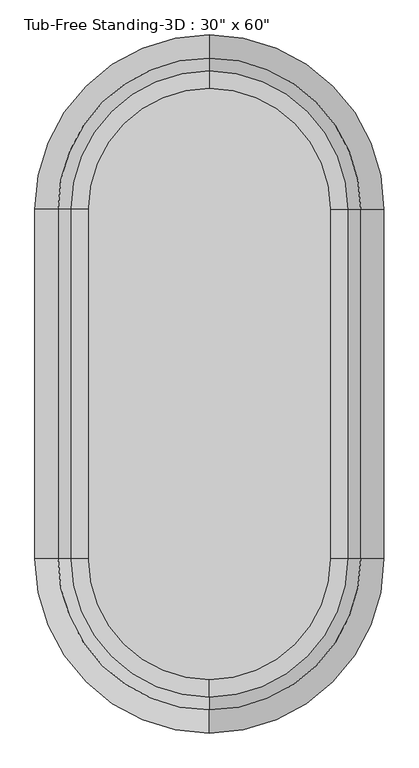
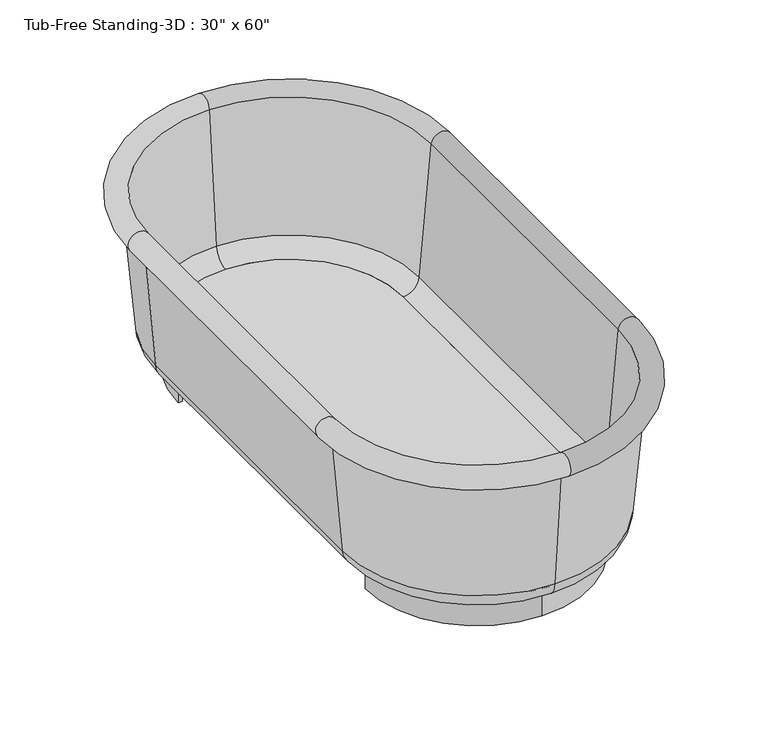
"""IFC4 building model written with IfcOpenShell, lengths in millimetres: flow terminal geometry."""

from ifc_helpers import new_model, si_unit, point, frame, frame_2d, origin, origin_with_axes, place, context, project, spatial, polyline, circle_curve, ellipse_curve, trimmed, segment, composite_curve, outline, extrude, source, transform, mapped, element, save
from ifc_brep_helpers import plane_surface, cylinder_surface, revolved_surface, advanced_brep


def flow_terminal_0c5ffde2(model_context):
    return source(origin(), model_context, "Body", "SolidModel", [
        advanced_brep(
        [(0.0, -723.9, 406.4), (342.9, -381.0, 406.4), (355.6, -381.0, 406.4), (0.0, -736.6, 406.4), (0.0, -698.1045038, 111.5561295), (317.1045038, -381.0, 111.5561295), (0.0, -645.2824236, 63.1536107), (264.2824236, -381.0, 63.1536107), (0.0, -645.2824236, 78.0774627), (264.2824236, -381.0, 78.0774627), (0.0, -683.2374416, 112.8568289), (302.2374416, -381.0, 112.8568289), (0.0, -711.4561556, 435.3982063), (330.4561556, -381.0, 435.3982063), (-342.9, -381.0, 406.4), (-355.6, -381.0, 406.4), (-317.1045038, -381.0, 111.5561295), (-264.2824236, -381.0, 63.1536107), (-264.2824236, -381.0, 78.0774627), (-302.2374416, -381.0, 112.8568289), (-330.4561556, -381.0, 435.3982063), (-355.6, 381.0, 406.4), (-342.9, 381.0, 406.4), (-317.1045038, 381.0, 111.5561295), (-264.2824236, 381.0, 63.1536107), (-264.2824236, 381.0, 78.0774627), (-302.2374416, 381.0, 112.8568289), (-330.4561556, 381.0, 435.3982063), (0.0, 723.9, 406.4), (0.0, 736.6, 406.4), (0.0, 698.1045038, 111.5561295), (0.0, 645.2824236, 63.1536107), (0.0, 645.2824236, 78.0774627), (0.0, 683.2374416, 112.8568289), (0.0, 711.4561556, 435.3982063), (342.9, 381.0, 406.4), (355.6, 381.0, 406.4), (317.1045038, 381.0, 111.5561295), (264.2824236, 381.0, 63.1536107), (264.2824236, 381.0, 78.0774627), (302.2374416, 381.0, 112.8568289), (330.4561556, 381.0, 435.3982063)],
        [
            (0, 1, circle_curve(frame((0.0, -381.0, 406.4), z_axis=(0.0, 0.0, 1.0), x_axis=(1.0, 0.0, 0.0)), 342.9)),
            (1, 2),
            (2, 3, circle_curve(frame((0.0, -381.0, 406.4), z_axis=(0.0, 0.0, -1.0), x_axis=(1.0, 0.0, 0.0)), 355.6)),
            (3, 0),
            (4, 5, circle_curve(frame((0.0, -381.0, 111.5561295), z_axis=(0.0, 0.0, 1.0), x_axis=(1.0, 0.0, 0.0)), 317.1045038)),
            (5, 1),
            (0, 4),
            (6, 7, circle_curve(frame((0.0, -381.0, 63.1536107), z_axis=(0.0, 0.0, 1.0), x_axis=(1.0, 0.0, 0.0)), 264.2824236)),
            (7, 5, circle_curve(frame((264.2824236, -381.0, 116.1774627), z_axis=(0.0, -1.0, 0.0), x_axis=(1.0, 0.0, 0.0)), 53.023852)),
            (4, 6, circle_curve(frame((0.0, -645.2824236, 116.1774627), z_axis=(1.0, 0.0, 0.0), x_axis=(0.0, -1.0, 0.0)), 53.023852)),
            (8, 9, circle_curve(frame((0.0, -381.0, 78.0774627), z_axis=(0.0, 0.0, 1.0), x_axis=(1.0, 0.0, 0.0)), 264.2824236)),
            (9, 7),
            (6, 8),
            (10, 11, circle_curve(frame((0.0, -381.0, 112.8568289), z_axis=(0.0, 0.0, 1.0), x_axis=(1.0, 0.0, 0.0)), 302.2374416)),
            (11, 9, circle_curve(frame((264.2824236, -381.0, 116.1774627), z_axis=(0.0, 1.0, 0.0), x_axis=(1.0, 0.0, 0.0)), 38.1)),
            (8, 10, circle_curve(frame((0.0, -645.2824236, 116.1774627), z_axis=(-1.0, 0.0, 0.0), x_axis=(0.0, -1.0, 0.0)), 38.1)),
            (12, 13, circle_curve(frame((0.0, -381.0, 435.3982063), z_axis=(0.0, 0.0, 1.0), x_axis=(1.0, 0.0, 0.0)), 330.4561556)),
            (13, 11),
            (10, 12),
            (2, 13, circle_curve(frame((355.6, -381.0, 431.8), z_axis=(0.0, -1.0, 0.0), x_axis=(1.0, 0.0, 0.0)), 25.4)),
            (12, 3, circle_curve(frame((0.0, -736.6, 431.8), z_axis=(1.0, 0.0, 0.0), x_axis=(0.0, -1.0, 0.0)), 25.4)),
            (14, 0, circle_curve(frame((0.0, -381.0, 406.4), z_axis=(0.0, 0.0, 1.0), x_axis=(0.0, -1.0, 0.0)), 342.9)),
            (3, 15, circle_curve(frame((0.0, -381.0, 406.4), z_axis=(0.0, 0.0, -1.0), x_axis=(0.0, -1.0, 0.0)), 355.6)),
            (15, 14),
            (16, 4, circle_curve(frame((0.0, -381.0, 111.5561295), z_axis=(0.0, 0.0, 1.0), x_axis=(0.0, -1.0, 0.0)), 317.1045038)),
            (14, 16),
            (17, 6, circle_curve(frame((0.0, -381.0, 63.1536107), z_axis=(0.0, 0.0, 1.0), x_axis=(0.0, -1.0, 0.0)), 264.2824236)),
            (16, 17, circle_curve(frame((-264.2824236, -381.0, 116.1774627), z_axis=(0.0, -1.0, 0.0), x_axis=(-1.0, 0.0, 0.0)), 53.023852)),
            (18, 8, circle_curve(frame((0.0, -381.0, 78.0774627), z_axis=(0.0, 0.0, 1.0), x_axis=(0.0, -1.0, 0.0)), 264.2824236)),
            (17, 18),
            (19, 10, circle_curve(frame((0.0, -381.0, 112.8568289), z_axis=(0.0, 0.0, 1.0), x_axis=(0.0, -1.0, 0.0)), 302.2374416)),
            (18, 19, circle_curve(frame((-264.2824236, -381.0, 116.1774627), z_axis=(0.0, 1.0, 0.0), x_axis=(-1.0, 0.0, 0.0)), 38.1)),
            (20, 12, circle_curve(frame((0.0, -381.0, 435.3982063), z_axis=(0.0, 0.0, 1.0), x_axis=(0.0, -1.0, 0.0)), 330.4561556)),
            (19, 20),
            (20, 15, circle_curve(frame((-355.6, -381.0, 431.8), z_axis=(0.0, -1.0, 0.0), x_axis=(-1.0, 0.0, 0.0)), 25.4)),
            (15, 21),
            (21, 22),
            (22, 14),
            (22, 23),
            (23, 16),
            (23, 24, circle_curve(frame((-264.2824236, 381.0, 116.1774627), z_axis=(0.0, -1.0, 0.0), x_axis=(-1.0, 0.0, 0.0)), 53.023852)),
            (24, 17),
            (24, 25),
            (25, 18),
            (25, 26, circle_curve(frame((-264.2824236, 381.0, 116.1774627), z_axis=(0.0, 1.0, 0.0), x_axis=(-1.0, 0.0, 0.0)), 38.1)),
            (26, 19),
            (26, 27),
            (27, 20),
            (27, 21, circle_curve(frame((-355.6, 381.0, 431.8), z_axis=(0.0, -1.0, 0.0), x_axis=(-1.0, 0.0, 0.0)), 25.4)),
            (28, 22, circle_curve(frame((0.0, 381.0, 406.4), z_axis=(0.0, 0.0, 1.0), x_axis=(-1.0, 0.0, 0.0)), 342.9)),
            (21, 29, circle_curve(frame((0.0, 381.0, 406.4), z_axis=(0.0, 0.0, -1.0), x_axis=(-1.0, 0.0, 0.0)), 355.6)),
            (29, 28),
            (30, 23, circle_curve(frame((0.0, 381.0, 111.5561295), z_axis=(0.0, 0.0, 1.0), x_axis=(-1.0, 0.0, 0.0)), 317.1045038)),
            (28, 30),
            (31, 24, circle_curve(frame((0.0, 381.0, 63.1536107), z_axis=(0.0, 0.0, 1.0), x_axis=(-1.0, 0.0, 0.0)), 264.2824236)),
            (30, 31, circle_curve(frame((0.0, 645.2824236, 116.1774627), z_axis=(-1.0, 0.0, 0.0), x_axis=(0.0, 1.0, 0.0)), 53.023852)),
            (32, 25, circle_curve(frame((0.0, 381.0, 78.0774627), z_axis=(0.0, 0.0, 1.0), x_axis=(-1.0, 0.0, 0.0)), 264.2824236)),
            (31, 32),
            (33, 26, circle_curve(frame((0.0, 381.0, 112.8568289), z_axis=(0.0, 0.0, 1.0), x_axis=(-1.0, 0.0, 0.0)), 302.2374416)),
            (32, 33, circle_curve(frame((0.0, 645.2824236, 116.1774627), z_axis=(1.0, 0.0, 0.0), x_axis=(0.0, 1.0, 0.0)), 38.1)),
            (34, 27, circle_curve(frame((0.0, 381.0, 435.3982063), z_axis=(0.0, 0.0, 1.0), x_axis=(-1.0, 0.0, 0.0)), 330.4561556)),
            (33, 34),
            (34, 29, circle_curve(frame((0.0, 736.6, 431.8), z_axis=(-1.0, 0.0, 0.0), x_axis=(0.0, 1.0, 0.0)), 25.4)),
            (35, 28, circle_curve(frame((0.0, 381.0, 406.4), z_axis=(0.0, 0.0, 1.0), x_axis=(0.0, 1.0, 0.0)), 342.9)),
            (29, 36, circle_curve(frame((0.0, 381.0, 406.4), z_axis=(0.0, 0.0, -1.0), x_axis=(0.0, 1.0, 0.0)), 355.6)),
            (36, 35),
            (37, 30, circle_curve(frame((0.0, 381.0, 111.5561295), z_axis=(0.0, 0.0, 1.0), x_axis=(0.0, 1.0, 0.0)), 317.1045038)),
            (35, 37),
            (38, 31, circle_curve(frame((0.0, 381.0, 63.1536107), z_axis=(0.0, 0.0, 1.0), x_axis=(0.0, 1.0, 0.0)), 264.2824236)),
            (37, 38, circle_curve(frame((264.2824236, 381.0, 116.1774627), z_axis=(0.0, 1.0, 0.0), x_axis=(1.0, 0.0, 0.0)), 53.023852)),
            (39, 32, circle_curve(frame((0.0, 381.0, 78.0774627), z_axis=(0.0, 0.0, 1.0), x_axis=(0.0, 1.0, 0.0)), 264.2824236)),
            (38, 39),
            (40, 33, circle_curve(frame((0.0, 381.0, 112.8568289), z_axis=(0.0, 0.0, 1.0), x_axis=(0.0, 1.0, 0.0)), 302.2374416)),
            (39, 40, circle_curve(frame((264.2824236, 381.0, 116.1774627), z_axis=(0.0, -1.0, 0.0), x_axis=(1.0, 0.0, 0.0)), 38.1)),
            (41, 34, circle_curve(frame((0.0, 381.0, 435.3982063), z_axis=(0.0, 0.0, 1.0), x_axis=(0.0, 1.0, 0.0)), 330.4561556)),
            (40, 41),
            (41, 36, circle_curve(frame((355.6, 381.0, 431.8), z_axis=(0.0, 1.0, 0.0), x_axis=(1.0, 0.0, 0.0)), 25.4)),
            (36, 2),
            (1, 35),
            (5, 37),
            (7, 38),
            (9, 39),
            (11, 40),
            (13, 41),
        ],
        [
            plane_surface(frame((0.0, -381.0, 406.4), z_axis=(0.0, 0.0, -1.0), x_axis=(1.0, 0.0, 0.0))),
            revolved_surface(polyline([(342.9, -381.0, 406.4), (317.1045038, -381.0, 111.5561295)]), (0.0, -381.0, 431.8), (0.0, 0.0, -1.0)),
            revolved_surface(trimmed(ellipse_curve(frame((264.2824236, -381.0, 116.1774627), z_axis=(0.0, 1.0, 0.0), x_axis=(1.0, 0.0, 0.0)), 53.023852, 53.023852), [point((317.1045038, -381.0, 111.5561295))], [point((264.2824236, -381.0, 63.1536107))], True, "CARTESIAN"), (0.0, -381.0, 431.8), (0.0, 0.0, -1.0)),
            revolved_surface(polyline([(264.2824236, -381.0, 63.1536107), (264.2824236, -381.0, 78.07746270000001)]), (0.0, -381.0, 431.8), (0.0, 0.0, -1.0)),
            revolved_surface(trimmed(ellipse_curve(frame((264.2824236, -381.0, 116.1774627), z_axis=(0.0, -1.0, 0.0), x_axis=(1.0, 0.0, 0.0)), 38.1, 38.1), [point((264.2824236, -381.0, 78.0774627))], [point((302.2374416, -381.0, 112.8568289))], True, "CARTESIAN"), (0.0, -381.0, 431.8), (0.0, 0.0, -1.0)),
            revolved_surface(polyline([(302.2374416, -381.0, 112.8568289), (330.4561556, -381.0, 435.3982063)]), (0.0, -381.0, 431.8), (0.0, 0.0, -1.0)),
            revolved_surface(trimmed(ellipse_curve(frame((355.6, -381.0, 431.8), z_axis=(0.0, 1.0, 0.0), x_axis=(1.0, 0.0, 0.0)), 25.4, 25.4), [point((330.4561556, -381.0, 435.3982063))], [point((355.6, -381.0, 406.4))], True, "CARTESIAN"), (0.0, -381.0, 431.8), (0.0, 0.0, -1.0)),
            plane_surface(frame((0.0, -381.0, 406.4), z_axis=(0.0, 0.0, -1.0), x_axis=(0.0, -1.0, 0.0))),
            revolved_surface(polyline([(0.0, -723.9, 406.4), (0.0, -698.1045038, 111.5561295)]), (0.0, -381.0, 431.8), (0.0, 0.0, -1.0)),
            revolved_surface(trimmed(ellipse_curve(frame((0.0, -645.2824236, 116.1774627), z_axis=(1.0, 0.0, 0.0), x_axis=(0.0, -1.0, 0.0)), 53.023852, 53.023852), [point((0.0, -698.1045038, 111.5561295))], [point((0.0, -645.2824236, 63.1536107))], True, "CARTESIAN"), (0.0, -381.0, 431.8), (0.0, 0.0, -1.0)),
            revolved_surface(polyline([(0.0, -645.2824236, 63.1536107), (0.0, -645.2824236, 78.07746270000001)]), (0.0, -381.0, 431.8), (0.0, 0.0, -1.0)),
            revolved_surface(trimmed(ellipse_curve(frame((0.0, -645.2824236, 116.1774627), z_axis=(-1.0, 0.0, 0.0), x_axis=(0.0, -1.0, 0.0)), 38.1, 38.1), [point((0.0, -645.2824236, 78.0774627))], [point((0.0, -683.2374416, 112.8568289))], True, "CARTESIAN"), (0.0, -381.0, 431.8), (0.0, 0.0, -1.0)),
            revolved_surface(polyline([(0.0, -683.2374416, 112.8568289), (0.0, -711.4561556, 435.3982063)]), (0.0, -381.0, 431.8), (0.0, 0.0, -1.0)),
            revolved_surface(trimmed(ellipse_curve(frame((0.0, -736.6, 431.8), z_axis=(1.0, 0.0, 0.0), x_axis=(0.0, -1.0, 0.0)), 25.4, 25.4), [point((0.0, -711.4561556, 435.3982063))], [point((0.0, -736.6, 406.4))], True, "CARTESIAN"), (0.0, -381.0, 431.8), (0.0, 0.0, -1.0)),
            plane_surface(frame((-355.6, -381.0, 406.4), z_axis=(0.0, 0.0, -1.0), x_axis=(0.0, 1.0, 0.0))),
            plane_surface(frame((-342.9, -381.0, 406.4), z_axis=(-0.9961946980917455, 0.0, -0.08715574274765871), x_axis=(0.0, 1.0, 0.0))),
            cylinder_surface(frame((-264.2824236, -381.0, 116.1774627), z_axis=(0.0, -1.0, 0.0), x_axis=(-1.0, 0.0, 0.0)), 53.023852),
            plane_surface(frame((-264.2824236, -381.0, 63.1536107), z_axis=(1.0, 0.0, 0.0), x_axis=(0.0, 1.0, 0.0))),
            revolved_surface(polyline([(-302.38242360000004, 381.0, 116.1774627), (-302.38242360000004, -381.0, 116.1774627)]), (-264.2824236, -381.0, 116.1774627), (0.0, 1.0, 0.0)),
            plane_surface(frame((-302.2374416, -381.0, 112.8568289), z_axis=(0.9961946980917458, 0.0, 0.08715574274765651), x_axis=(0.0, 1.0, 0.0))),
            cylinder_surface(frame((-355.6, -381.0, 431.8), z_axis=(0.0, -1.0, 0.0), x_axis=(-1.0, 0.0, 0.0)), 25.4),
            plane_surface(frame((0.0, 381.0, 406.4), z_axis=(0.0, 0.0, -1.0), x_axis=(-1.0, 0.0, 0.0))),
            revolved_surface(polyline([(-342.9, 381.0, 406.4), (-317.1045038, 381.0, 111.5561295)]), (0.0, 381.0, 431.8), (0.0, 0.0, -1.0)),
            revolved_surface(trimmed(ellipse_curve(frame((-264.2824236, 381.0, 116.1774627), z_axis=(0.0, -1.0, 0.0), x_axis=(-1.0, 0.0, 0.0)), 53.023852, 53.023852), [point((-317.1045038, 381.0, 111.5561295))], [point((-264.2824236, 381.0, 63.1536107))], True, "CARTESIAN"), (0.0, 381.0, 431.8), (0.0, 0.0, -1.0)),
            revolved_surface(polyline([(-264.2824236, 381.0, 63.1536107), (-264.2824236, 381.0, 78.07746270000001)]), (0.0, 381.0, 431.8), (0.0, 0.0, -1.0)),
            revolved_surface(trimmed(ellipse_curve(frame((-264.2824236, 381.0, 116.1774627), z_axis=(0.0, 1.0, 0.0), x_axis=(-1.0, 0.0, 0.0)), 38.1, 38.1), [point((-264.2824236, 381.0, 78.0774627))], [point((-302.2374416, 381.0, 112.8568289))], True, "CARTESIAN"), (0.0, 381.0, 431.8), (0.0, 0.0, -1.0)),
            revolved_surface(polyline([(-302.2374416, 381.0, 112.8568289), (-330.4561556, 381.0, 435.3982063)]), (0.0, 381.0, 431.8), (0.0, 0.0, -1.0)),
            revolved_surface(trimmed(ellipse_curve(frame((-355.6, 381.0, 431.8), z_axis=(0.0, -1.0, 0.0), x_axis=(-1.0, 0.0, 0.0)), 25.4, 25.4), [point((-330.4561556, 381.0, 435.3982063))], [point((-355.6, 381.0, 406.4))], True, "CARTESIAN"), (0.0, 381.0, 431.8), (0.0, 0.0, -1.0)),
            plane_surface(frame((0.0, 381.0, 406.4), z_axis=(0.0, 0.0, -1.0), x_axis=(0.0, 1.0, 0.0))),
            revolved_surface(polyline([(0.0, 723.9, 406.4), (0.0, 698.1045038, 111.5561295)]), (0.0, 381.0, 431.8), (0.0, 0.0, -1.0)),
            revolved_surface(trimmed(ellipse_curve(frame((0.0, 645.2824236, 116.1774627), z_axis=(-1.0, 0.0, 0.0), x_axis=(0.0, 1.0, 0.0)), 53.023852, 53.023852), [point((0.0, 698.1045038, 111.5561295))], [point((0.0, 645.2824236, 63.1536107))], True, "CARTESIAN"), (0.0, 381.0, 431.8), (0.0, 0.0, -1.0)),
            revolved_surface(polyline([(0.0, 645.2824236, 63.1536107), (0.0, 645.2824236, 78.07746270000001)]), (0.0, 381.0, 431.8), (0.0, 0.0, -1.0)),
            revolved_surface(trimmed(ellipse_curve(frame((0.0, 645.2824236, 116.1774627), z_axis=(1.0, 0.0, 0.0), x_axis=(0.0, 1.0, 0.0)), 38.1, 38.1), [point((0.0, 645.2824236, 78.0774627))], [point((0.0, 683.2374416, 112.8568289))], True, "CARTESIAN"), (0.0, 381.0, 431.8), (0.0, 0.0, -1.0)),
            revolved_surface(polyline([(0.0, 683.2374416, 112.8568289), (0.0, 711.4561556, 435.3982063)]), (0.0, 381.0, 431.8), (0.0, 0.0, -1.0)),
            revolved_surface(trimmed(ellipse_curve(frame((0.0, 736.6, 431.8), z_axis=(-1.0, 0.0, 0.0), x_axis=(0.0, 1.0, 0.0)), 25.4, 25.4), [point((0.0, 711.4561556, 435.3982063))], [point((0.0, 736.6, 406.4))], True, "CARTESIAN"), (0.0, 381.0, 431.8), (0.0, 0.0, -1.0)),
            plane_surface(frame((355.6, 381.0, 406.4), z_axis=(0.0, 0.0, -1.0), x_axis=(0.0, -1.0, 0.0))),
            plane_surface(frame((342.9, 381.0, 406.4), z_axis=(0.9961946980917455, 0.0, -0.08715574274765871), x_axis=(0.0, -1.0, 0.0))),
            cylinder_surface(frame((264.2824236, 381.0, 116.1774627), z_axis=(0.0, 1.0, 0.0), x_axis=(1.0, 0.0, 0.0)), 53.023852),
            plane_surface(frame((264.2824236, 381.0, 63.1536107), z_axis=(-1.0, 0.0, 0.0), x_axis=(0.0, -1.0, 0.0))),
            revolved_surface(polyline([(302.38242360000004, -381.0, 116.1774627), (302.38242360000004, 381.0, 116.1774627)]), (264.2824236, 381.0, 116.1774627), (0.0, -1.0, 0.0)),
            plane_surface(frame((302.2374416, 381.0, 112.8568289), z_axis=(-0.9961946980917458, 0.0, 0.08715574274765651), x_axis=(0.0, -1.0, 0.0))),
            cylinder_surface(frame((355.6, 381.0, 431.8), z_axis=(0.0, 1.0, 0.0), x_axis=(1.0, 0.0, 0.0)), 25.4),
        ],
        [
            (0, [[1, 2, 3, 4]]),
            (1, [[5, 6, -1, 7]]),
            (2, [[8, 9, -5, 10]]),
            (3, [[11, 12, -8, 13]]),
            (4, [[14, 15, -11, 16]]),
            (5, [[17, 18, -14, 19]]),
            (6, [[-3, 20, -17, 21]]),
            (7, [[22, -4, 23, 24]]),
            (8, [[25, -7, -22, 26]]),
            (9, [[27, -10, -25, 28]]),
            (10, [[29, -13, -27, 30]]),
            (11, [[31, -16, -29, 32]]),
            (12, [[33, -19, -31, 34]]),
            (13, [[-23, -21, -33, 35]]),
            (14, [[-24, 36, 37, 38]]),
            (15, [[-26, -38, 39, 40]]),
            (16, [[-28, -40, 41, 42]]),
            (17, [[-30, -42, 43, 44]]),
            (18, [[-32, -44, 45, 46]]),
            (19, [[-34, -46, 47, 48]]),
            (20, [[-35, -48, 49, -36]]),
            (21, [[50, -37, 51, 52]]),
            (22, [[53, -39, -50, 54]]),
            (23, [[55, -41, -53, 56]]),
            (24, [[57, -43, -55, 58]]),
            (25, [[59, -45, -57, 60]]),
            (26, [[61, -47, -59, 62]]),
            (27, [[-51, -49, -61, 63]]),
            (28, [[64, -52, 65, 66]]),
            (29, [[67, -54, -64, 68]]),
            (30, [[69, -56, -67, 70]]),
            (31, [[71, -58, -69, 72]]),
            (32, [[73, -60, -71, 74]]),
            (33, [[75, -62, -73, 76]]),
            (34, [[-65, -63, -75, 77]]),
            (35, [[-66, 78, -2, 79]]),
            (36, [[-68, -79, -6, 80]]),
            (37, [[-70, -80, -9, 81]]),
            (38, [[-72, -81, -12, 82]]),
            (39, [[-74, -82, -15, 83]]),
            (40, [[-76, -83, -18, 84]]),
            (41, [[-77, -84, -20, -78]]),
        ],
    ),
        extrude(outline(composite_curve([segment(polyline([(-264.2824236, -381.0), (-264.2824236, 381.0)]), True, "CONTINUOUS"), segment(trimmed(circle_curve(frame_2d((0.0, 381.0)), 264.2824236), [point((-264.2824236, 381.0))], [point((0.0, 645.2824236))], False, "CARTESIAN"), True, "CONTINUOUS"), segment(trimmed(circle_curve(frame_2d((0.0, 381.0)), 264.2824236), [point((0.0, 645.2824236))], [point((264.2824236, 381.0))], False, "CARTESIAN"), True, "CONTINUOUS"), segment(polyline([(264.2824236, 381.0), (264.2824236, -381.0)]), True, "CONTINUOUS"), segment(trimmed(circle_curve(frame_2d((0.0, -381.0)), 264.2824236), [point((264.2824236, -381.0))], [point((0.0, -645.2824236))], False, "CARTESIAN"), True, "CONTINUOUS"), segment(trimmed(circle_curve(frame_2d((0.0, -381.0)), 264.2824236), [point((0.0, -645.2824236))], [point((-264.2824236, -381.0))], False, "CARTESIAN"), True, "CONTINUOUS")], self_intersect=False)), frame((0.0, 0.0, 63.5), z_axis=(0.0, 0.0, 1.0), x_axis=(1.0, 0.0, 0.0)), (0.0, 0.0, 1.0), 15.08125),
        extrude(outline(composite_curve([segment(trimmed(circle_curve(frame_2d((0.0, -381.0)), 264.2824236), [point((0.0, -645.2824236))], [point((-264.2824236, -381.0))], False, "CARTESIAN"), True, "CONTINUOUS"), segment(polyline([(-264.2824236, -381.0), (-254.0, -381.0)]), True, "CONTINUOUS"), segment(trimmed(circle_curve(frame_2d((0.0, -381.0)), 254.0), [point((-254.0, -381.0))], [point((0.0, -635.0))], True, "CARTESIAN"), True, "CONTINUOUS"), segment(trimmed(circle_curve(frame_2d((0.0, -381.0)), 254.0), [point((0.0, -635.0))], [point((254.0, -381.0))], True, "CARTESIAN"), True, "CONTINUOUS"), segment(polyline([(254.0, -381.0), (264.2824236, -381.0)]), True, "CONTINUOUS"), segment(trimmed(circle_curve(frame_2d((0.0, -381.0)), 264.2824236), [point((264.2824236, -381.0))], [point((0.0, -645.2824236))], False, "CARTESIAN"), True, "CONTINUOUS")], self_intersect=False)), origin_with_axes(), (0.0, 0.0, 1.0), 63.5),
        extrude(outline(composite_curve([segment(trimmed(circle_curve(frame_2d((0.0, 381.0)), 254.0), [point((0.0, 635.0))], [point((-254.0, 381.0))], True, "CARTESIAN"), True, "CONTINUOUS"), segment(polyline([(-254.0, 381.0), (-264.2824236, 381.0)]), True, "CONTINUOUS"), segment(trimmed(circle_curve(frame_2d((0.0, 381.0)), 264.2824236), [point((-264.2824236, 381.0))], [point((0.0, 645.2824236))], False, "CARTESIAN"), True, "CONTINUOUS"), segment(trimmed(circle_curve(frame_2d((0.0, 381.0)), 264.2824236), [point((0.0, 645.2824236))], [point((264.2824236, 381.0))], False, "CARTESIAN"), True, "CONTINUOUS"), segment(polyline([(264.2824236, 381.0), (254.0, 381.0)]), True, "CONTINUOUS"), segment(trimmed(circle_curve(frame_2d((0.0, 381.0)), 254.0), [point((254.0, 381.0))], [point((0.0, 635.0))], True, "CARTESIAN"), True, "CONTINUOUS")], self_intersect=False)), origin_with_axes(), (0.0, 0.0, 1.0), 63.5),
    ])


if __name__ == "__main__":
    model = new_model("IFC4")
    model_context = context("Model", 3, world=origin())
    ifc_project = project(units=[si_unit("LENGTHUNIT", "METRE", prefix="MILLI")], contexts=[model_context])
    site = spatial("IfcSite", under=ifc_project)
    building = spatial("IfcBuilding", under=site)
    placement = place(None, origin())
    flow_terminal_shape = flow_terminal_0c5ffde2(model_context)
    element("IfcFlowTerminal", 1, ObjectType="Tub-Free Standing-3D : 30\" x 60\"", at=placement, inside=building, context=model_context, shape_type="MappedRepresentation", body=[
        mapped(flow_terminal_shape, transform((0.0, 0.0, 0.0), x_axis=(1.0, 0.0, 0.0), y_axis=(0.0, 1.0, 0.0), z_axis=(0.0, 0.0, 1.0))),
    ])
    save(model, "model.ifc")

# Revit data of these elements
# Type "Tub-Free Standing-3D : 30\" x 60\""
#   Assembly Code = "D2010110"
#   Height = 457.2 mm
#   Length = 1524 mm
#   Width = 762 mm
#   Tub Material = Porcelain, Ivory
#   Default Elevation = 0
# Element 1 (IfcFlowTerminal, "Tub-Free Standing-3D : 30\" x 60\"")
#   Materials on its faces: "Porcelain, Ivory"
# Materials
#   "Porcelain, Ivory": class "Ceramic", colour RGB 247 247 239, transparency 0, Description = "Porcelain, ivory", Cost = 0
